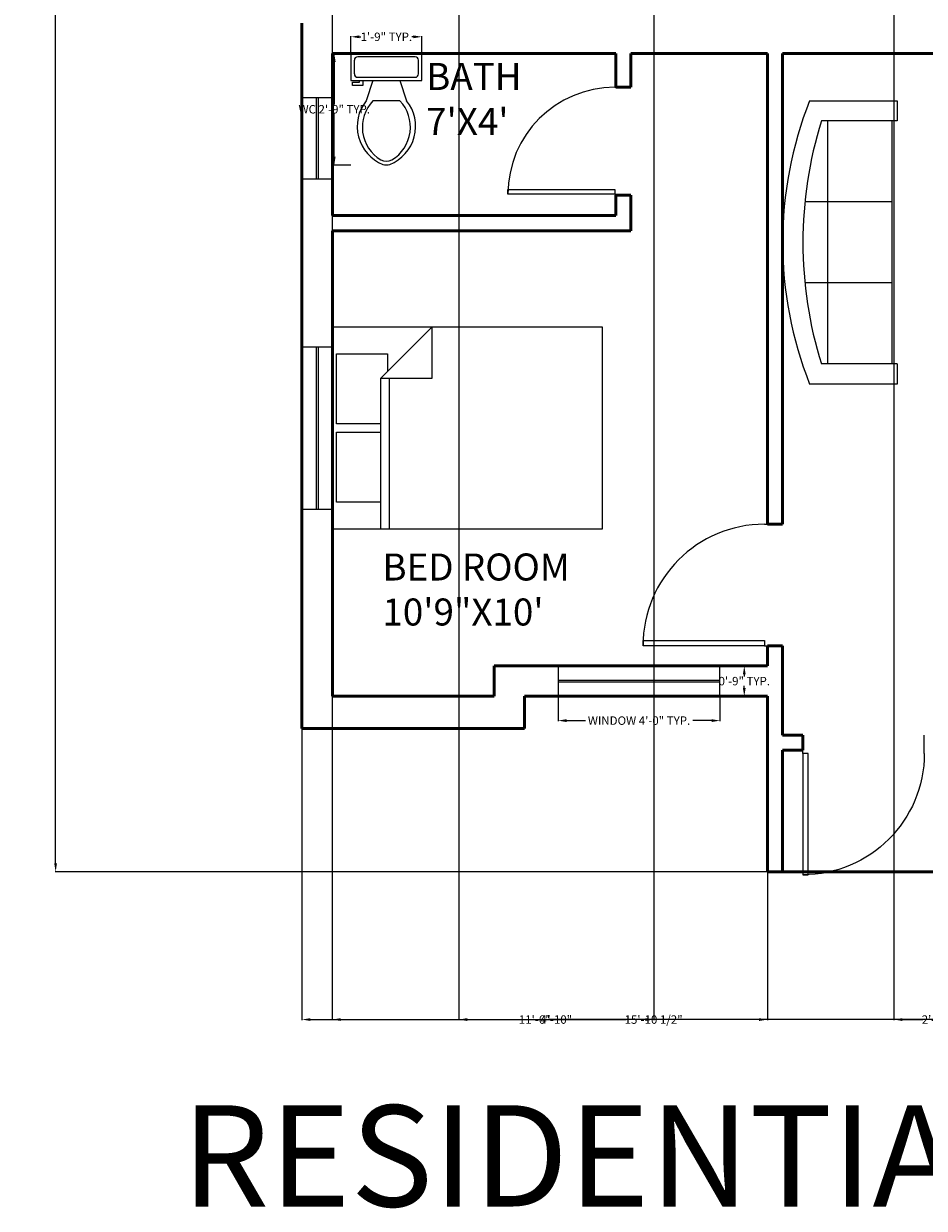
# Model space of a CAD drawing. Units: inches. Extents: x -46 to 565, y -56 to 809.
# Tile 1 of 6: x -46 to 221, y -56 to 296. Entities that reach past the tile are written whole.
import ezdxf

# ---------------------------------------------------------------- set-up
doc = ezdxf.new("R2010")
doc.units = ezdxf.units.IN
doc.header["$MEASUREMENT"] = 0
for name, color, linetype, lineweight in [('A-ANNO-DIMS', 2, 'Continuous', 18), ('A-ANNO-TEXT', 241, 'Continuous', 30), ('A-AREA-IDEN', 241, 'Continuous', 18), ('A-FLOR-FIXT', 131, 'Continuous', 18), ('A-FURN', 131, 'Continuous', 18), ('DOOR', 210, 'Continuous', 25), ('WALL', 10, 'Continuous', 50), ('WINDOW', 170, 'Continuous', 18)]:
    doc.layers.add(name, color=color, linetype=linetype, lineweight=lineweight)
doc.styles.get("Standard").update_dxf_attribs({"font": 'arial.ttf'})
doc.dimstyles.get("Standard").update_dxf_attribs({"dimtxt": 2.5, "dimasz": 2.5, "dimexe": 0.18, "dimexo": 0.0625, "dimgap": 0.09, "dimtad": 0, "dimtih": 1, "dimtoh": 1, "dimzin": 0, "dimdsep": 46, "dimlunit": 3, "dimtxsty": 'Standard', "dimcen": 0.09, "dimadec": 0, "dimazin": 0, "dimtfac": 1, "dimtofl": 0, "dimtmove": 0, "dimatfit": 3, "dimfxl": 1, "dimtolj": 1, "dimtzin": 0, "dimarcsym": 0})

# ---------------------------------------------------------------- blocks, each defined once
blk = doc.blocks.new('*U2')
for p, q in [((0, 0), (0, -6)), ((40, 0), (40, -6))]:
    blk.add_line(p, q)
blk.add_lwpolyline([(0, 0), (0, 40), (1.75, 40), (1.75, 0)], close=True)
blk.add_arc((0, 0), 40, 0, 90)
blk = doc.blocks.new('Bed - Queen')
for p, q in [((0, -80.00003), (0, 0)), ((0, 0), (59.99999, 0)), ((59.99999, 0), (59.99999, -80.00003)), ((7.99999, -1.2), (28.79998, -1.2)), ((7.99999, -14.4), (7.99999, -1.2)), ((28.79998, -1.2), (28.79998, -14.4)), ((31.19999, -1.2), (51.99999, -1.2)), ((31.19999, -14.4), (31.19999, -1.2)), ((51.99999, -1.2), (51.99999, -16.4)), ((0, -14.4), (44.8, -14.4)), ((44.8, -16.8), (0, -16.8)), ((59.99999, -29.6), (44.8, -14.4)), ((44.8, -14.4), (44.8, -29.6)), ((51.99999, -16.4), (46.79936, -16.4)), ((44.8, -29.6), (59.99999, -29.6)), ((59.99999, -80.00003), (0, -80.00003))]:
    blk.add_line(p, q)
blk = doc.blocks.new('Toilet - top')
for p, q in [((9.5, -6), (9.5, -2)), ((-10, -8.5), (-8, -8.5)), ((-10, -9.5), (-10, -8.5)), ((-7, -9.5), (-10, -9.5)), ((-8, -8.5), (-8, -8)), ((-7, -8), (-7, -9.5)), ((-4, -8), (-6, -14)), ((4, -8), (6, -14)), ((4, -14), (-4, -14))]:
    blk.add_line(p, q)
blk.add_lwpolyline([(10.5, -8), (10.5, 0), (-10.5, 0), (-10.5, -8)], close=True)
for points in [[(-9.5, -2), (-9.5, -6)], [(8.5, -1), (-8.5, -1)], [(-8.5, -7), (8.5, -7)]]:
    blk.add_lwpolyline(points)
for centre, radius, start, end in [((-8.62, -1.88), 0.884, 81.8699, 188.1301), ((8.62, -1.88), 0.884, 351.8699, 98.1301), ((-8.62, -6.12), 0.884, 171.8699, 278.1301), ((8.62, -6.12), 0.884, 261.8699, 8.1301), ((3.52, -21.58), 12.17, 141.4691, 247.9714), ((4.2, -21.82), 11.33, 136.3677, 238.9468), ((-3.52, -21.58), 12.17, 292.0284, 38.5307), ((-4.2, -21.82), 11.33, 301.053, 43.6321), ((0, -27.88), 4, 245.7318, 294.2682), ((0, -29), 4, 254.8605, 285.1395)]:
    blk.add_arc(centre, radius, start, end)
blk = doc.blocks.new('Sofa - Roundback 7 ft.')
for p, q in [((-12.00002, -32.4421), (-12.00003, -6.5971)), ((11.99997, -32.4421), (11.99998, -6.5971)), ((-36.000027, -34), (-36.000027, -11.4696)), ((-35.999844, -13.3819), (35.9998, -13.3819)), ((35.99998, -34), (35.99998, -11.4696)), ((-36.000027, -32.4421), (35.99998, -32.4421))]:
    blk.add_line(p, q)
for points in [[(-36.000027, -34), (-42.000027, -34), (-42.000027, -8)], [(41.99998, -8), (41.99998, -34), (35.99998, -34)]]:
    blk.add_lwpolyline(points)
for centre, radius, start, end in [((0, -114.25), 114.25, 68.43141, 111.5686), ((-0.00001, -127.1968), 121.1968, 72.72033, 107.2797)]:
    blk.add_arc(centre, radius, start, end)
blk = doc.blocks.new('*D15')
at = {"layer": 'A-ANNO-DIMS', "color": 0, "lineweight": -2, "transparency": 16777216}
for p, q in [((174.08, 764.2), (-37.07, 764.2)), ((-36.89, 761.7), (-36.89, 409.4)), ((-36.89, 46.7), (-36.89, 399)), ((174.08, 44.2), (-37.07, 44.2))]:
    blk.add_line(p, q, dxfattribs=at)
at = {"layer": 'A-ANNO-DIMS', "color": 0, "transparency": 16777216}
for points in [[(-37.31, 761.7), (-36.48, 761.7), (-36.89, 764.2)], [(-37.31, 46.7), (-36.48, 46.7), (-36.89, 44.2)]]:
    blk.add_solid(points, dxfattribs=at)
at = {"layer": 'Defpoints', "color": 0, "transparency": 16777216}
for p in [(-36.89, 764.2), (174.14, 764.2), (174.14, 44.2)]:
    blk.add_point(p, dxfattribs=at)
at = {"layer": 'A-ANNO-DIMS', "color": 0, "transparency": 16777216, "insert": (-36.89, 404.2), "char_height": 10, "attachment_point": 5}
blk.add_mtext("\\A1;60'", dxfattribs=at)
blk = doc.blocks.new('WIN-48IN')
for p, q in [((0, 4.75), (48, 4.75)), ((0, 4.25), (48, 4.25))]:
    blk.add_line(p, q)
blk.add_lwpolyline([(0, 0), (48, 0), (48, 9), (0, 9)], close=True)
blk = doc.blocks.new('WIN-24IN')
for p, q in [((4.25, 24), (4.25, 0)), ((4.75, 24), (4.75, 0))]:
    blk.add_line(p, q)
blk.add_lwpolyline([(0, 24), (0, 0), (9, 0), (9, 24)], close=True)
blk = doc.blocks.new('*D21')
at = {"layer": 'A-ANNO-DIMS', "color": 0, "lineweight": -2, "transparency": 16777216}
for p, q in [((50.6, 286.7), (45.53, 286.7)), ((45.71, 284.2), (45.71, 271.56)), ((45.71, 256.15), (45.71, 268.79)), ((50.6, 253.65), (45.53, 253.65))]:
    blk.add_line(p, q, dxfattribs=at)
at = {"layer": 'A-ANNO-DIMS', "color": 0, "transparency": 16777216}
for points in [[(45.29, 284.2), (46.12, 284.2), (45.71, 286.7)], [(45.29, 256.15), (46.12, 256.15), (45.71, 253.65)]]:
    blk.add_solid(points, dxfattribs=at)
at = {"layer": 'Defpoints', "color": 0, "transparency": 16777216}
for p in [(45.71, 286.7), (50.66, 286.7), (50.66, 253.65)]:
    blk.add_point(p, dxfattribs=at)
at = {"layer": 'A-ANNO-DIMS', "color": 0, "transparency": 16777216, "insert": (45.71, 270.18), "char_height": 2.5, "attachment_point": 5}
blk.add_mtext('\\A1;WC 2\'-9" TYP.', dxfattribs=at)
blk = doc.blocks.new('*D22')
at = {"layer": 'A-ANNO-DIMS', "color": 0, "lineweight": -2, "transparency": 16777216}
for p, q in [((50.66, 286.76), (50.66, 291.84)), ((53.16, 291.66), (53.57, 291.66)), ((69.16, 291.66), (68.75, 291.66)), ((71.66, 286.76), (71.66, 291.84))]:
    blk.add_line(p, q, dxfattribs=at)
at = {"layer": 'A-ANNO-DIMS', "color": 0, "transparency": 16777216}
for points in [[(53.16, 292.07), (53.16, 291.24), (50.66, 291.66)], [(69.16, 292.07), (69.16, 291.24), (71.66, 291.66)]]:
    blk.add_solid(points, dxfattribs=at)
at = {"layer": 'Defpoints', "color": 0, "transparency": 16777216}
for p in [(71.66, 291.66), (50.66, 286.7), (71.66, 286.7)]:
    blk.add_point(p, dxfattribs=at)
at = {"layer": 'A-ANNO-DIMS', "color": 0, "transparency": 16777216, "insert": (61.16, 291.66), "char_height": 2.5, "attachment_point": 5}
blk.add_mtext('\\A1;1\'-9" TYP.', dxfattribs=at)
blk = doc.blocks.new('*D23')
at = {"layer": 'A-ANNO-DIMS', "color": 0, "lineweight": -2, "transparency": 16777216}
for p, q in [((112.07, 96.14), (112.07, 88.82)), ((160.07, 96.14), (160.07, 88.82)), ((114.57, 89), (120.16, 89)), ((157.57, 89), (151.97, 89))]:
    blk.add_line(p, q, dxfattribs=at)
at = {"layer": 'A-ANNO-DIMS', "color": 0, "transparency": 16777216}
for points in [[(114.57, 89.42), (114.57, 88.58), (112.07, 89)], [(157.57, 89.42), (157.57, 88.58), (160.07, 89)]]:
    blk.add_solid(points, dxfattribs=at)
at = {"layer": 'Defpoints', "color": 0, "transparency": 16777216}
for p in [(112.07, 96.2), (160.07, 96.2), (160.07, 89)]:
    blk.add_point(p, dxfattribs=at)
at = {"layer": 'A-ANNO-DIMS', "color": 0, "transparency": 16777216, "insert": (136.07, 89), "char_height": 2.5, "attachment_point": 5}
blk.add_mtext('\\A1;WINDOW 4\'-0" TYP.', dxfattribs=at)
blk = doc.blocks.new('*D24')
at = {"layer": 'A-ANNO-DIMS', "color": 0, "lineweight": -2, "transparency": 16777216}
for p, q in [((160.13, 105.2), (167.45, 105.2)), ((167.27, 102.7), (167.27, 102.07)), ((167.27, 98.7), (167.27, 99.33)), ((160.13, 96.2), (167.45, 96.2))]:
    blk.add_line(p, q, dxfattribs=at)
at = {"layer": 'A-ANNO-DIMS', "color": 0, "transparency": 16777216}
for points in [[(166.85, 102.7), (167.68, 102.7), (167.27, 105.2)], [(166.85, 98.7), (167.68, 98.7), (167.27, 96.2)]]:
    blk.add_solid(points, dxfattribs=at)
at = {"layer": 'Defpoints', "color": 0, "transparency": 16777216}
for p in [(160.07, 105.2), (167.27, 105.2), (160.07, 96.2)]:
    blk.add_point(p, dxfattribs=at)
at = {"layer": 'A-ANNO-DIMS', "color": 0, "transparency": 16777216, "insert": (167.27, 100.7), "char_height": 2.5, "attachment_point": 5}
blk.add_mtext('\\A1;0\'-9" TYP.', dxfattribs=at)
blk = doc.blocks.new('*D48')
at = {"layer": 'A-ANNO-DIMS', "color": 0, "lineweight": -2, "transparency": 16777216}
for p, q in [((36.14, 86.62), (36.14, 0.22)), ((174.14, 44.14), (174.14, 0.22)), ((38.64, 0.4), (100.88, 0.4)), ((171.64, 0.4), (109.41, 0.4))]:
    blk.add_line(p, q, dxfattribs=at)
at = {"layer": 'A-ANNO-DIMS', "color": 0, "transparency": 16777216}
for points in [[(38.64, 0.82), (38.64, -0.02), (36.14, 0.4)], [(171.64, 0.82), (171.64, -0.02), (174.14, 0.4)]]:
    blk.add_solid(points, dxfattribs=at)
at = {"layer": 'Defpoints', "color": 0, "transparency": 16777216}
for p in [(36.14, 86.68), (174.14, 44.2), (174.14, 0.4)]:
    blk.add_point(p, dxfattribs=at)
at = {"layer": 'A-ANNO-DIMS', "color": 0, "transparency": 16777216, "insert": (105.14, 0.4), "char_height": 2.5, "attachment_point": 5}
blk.add_mtext('\\A1;11\'-6"', dxfattribs=at)
blk = doc.blocks.new('*D50')
at = {"layer": 'A-ANNO-DIMS', "color": 0, "lineweight": -2, "transparency": 16777216}
for p, q in [((211.64, 558.64), (211.64, 0.22)), ((235.64, 558.64), (235.64, 0.22)), ((214.14, 0.4), (220.21, 0.4)), ((233.14, 0.4), (227.08, 0.4))]:
    blk.add_line(p, q, dxfattribs=at)
at = {"layer": 'A-ANNO-DIMS', "color": 0, "transparency": 16777216}
for points in [[(214.14, 0.82), (214.14, -0.02), (211.64, 0.4)], [(233.14, 0.82), (233.14, -0.02), (235.64, 0.4)]]:
    blk.add_solid(points, dxfattribs=at)
at = {"layer": 'Defpoints', "color": 0, "transparency": 16777216}
for p in [(211.64, 558.7), (235.64, 558.7), (235.64, 0.4)]:
    blk.add_point(p, dxfattribs=at)
at = {"layer": 'A-ANNO-DIMS', "color": 0, "transparency": 16777216, "insert": (223.64, 0.4), "char_height": 2.5, "attachment_point": 5}
blk.add_mtext('\\A1;2\'-0"', dxfattribs=at)
blk = doc.blocks.new('*D51')
at = {"layer": 'A-ANNO-DIMS', "color": 0, "lineweight": -2, "transparency": 16777216}
for p, q in [((82.64, 554.14), (82.64, 0.22)), ((140.42, 554.14), (140.42, 0.22)), ((85.14, 0.4), (107.1, 0.4)), ((137.92, 0.4), (115.96, 0.4))]:
    blk.add_line(p, q, dxfattribs=at)
at = {"layer": 'A-ANNO-DIMS', "color": 0, "transparency": 16777216}
for points in [[(85.14, 0.82), (85.14, -0.02), (82.64, 0.4)], [(137.92, 0.82), (137.92, -0.02), (140.42, 0.4)]]:
    blk.add_solid(points, dxfattribs=at)
at = {"layer": 'Defpoints', "color": 0, "transparency": 16777216}
for p in [(82.64, 554.2), (140.42, 554.2), (140.42, 0.4)]:
    blk.add_point(p, dxfattribs=at)
at = {"layer": 'A-ANNO-DIMS', "color": 0, "transparency": 16777216, "insert": (111.53, 0.4), "char_height": 2.5, "attachment_point": 5}
blk.add_mtext('\\A1;4\'-10"', dxfattribs=at)
blk = doc.blocks.new('*D55')
at = {"layer": 'A-ANNO-DIMS', "color": 0, "lineweight": -2, "transparency": 16777216}
for p, q in [((45.14, 407.14), (45.14, 0.22)), ((235.64, 407.14), (235.64, 0.22)), ((47.64, 0.4), (132.24, 0.4)), ((233.14, 0.4), (148.54, 0.4))]:
    blk.add_line(p, q, dxfattribs=at)
at = {"layer": 'A-ANNO-DIMS', "color": 0, "transparency": 16777216}
for points in [[(47.64, 0.82), (47.64, -0.02), (45.14, 0.4)], [(233.14, 0.82), (233.14, -0.02), (235.64, 0.4)]]:
    blk.add_solid(points, dxfattribs=at)
at = {"layer": 'Defpoints', "color": 0, "transparency": 16777216}
for p in [(45.14, 407.2), (235.64, 407.2), (235.64, 0.4)]:
    blk.add_point(p, dxfattribs=at)
at = {"layer": 'A-ANNO-DIMS', "color": 0, "transparency": 16777216, "insert": (140.39, 0.4), "char_height": 2.5, "attachment_point": 5}
blk.add_mtext('\\A1;15\'-10 1/2"', dxfattribs=at)

msp = doc.modelspace()

# ---------------------------------------------------------------- linework, layer by layer
at = {"layer": 'WALL'}
for p, q in [((36.143, 295.7), (36.143, 86.684)), ((45.143, 286.7), (45.143, 238.7)), ((129.143, 286.7), (45.143, 286.7)), ((129.143, 286.7), (129.143, 276.7)), ((133.643, 286.7), (133.643, 276.7)), ((174.143, 286.7), (133.643, 286.7)), ((174.143, 286.7), (174.143, 147.2)), ((244.643, 286.7), (178.643, 286.7)), ((178.643, 286.7), (178.643, 147.2)), ((133.643, 276.7), (129.143, 276.7)), ((133.643, 244.7), (129.143, 244.7)), ((129.143, 244.7), (129.143, 238.7)), ((133.643, 244.7), (133.643, 234.2)), ((129.143, 238.7), (45.143, 238.7)), ((45.143, 234.2), (45.143, 114.2)), ((133.643, 234.2), (45.143, 234.2)), ((174.143, 147.2), (178.643, 147.2)), ((45.143, 114.2), (45.143, 96.2)), ((174.143, 111.2), (178.643, 111.2)), ((174.143, 111.2), (174.143, 105.2)), ((178.643, 111.2), (178.643, 96.2)), ((102.143, 105.2), (93.143, 105.2)), ((93.143, 105.2), (93.143, 96.2)), ((174.143, 105.2), (102.143, 105.2)), ((93.143, 96.2), (45.143, 96.2)), ((174.143, 96.2), (102.143, 96.2)), ((129.143, 96.2), (102.143, 96.2)), ((102.143, 96.2), (102.143, 86.684)), ((174.143, 44.2), (174.143, 96.2)), ((178.643, 96.2), (178.643, 84.7)), ((102.143, 86.684), (36.143, 86.684)), ((184.643, 84.7), (178.643, 84.7)), ((184.643, 84.7), (184.643, 80.2)), ((184.643, 80.2), (178.643, 80.2)), ((178.643, 80.2), (178.643, 44.2)), ((235.643, 44.2), (174.143, 44.2))]:
    msp.add_line(p, q, dxfattribs=at)

# ---------------------------------------------------------------- block references
at = {"layer": 'A-FLOR-FIXT'}
msp.add_blockref('Toilet - top', (61.163, 286.7), dxfattribs=at)
at = {"layer": 'A-FURN', "rotation": 90}
for name, p in [('Sofa - Roundback 7 ft.', (178.643, 230.706)), ('Bed - Queen', (45.143, 145.711))]:
    msp.add_blockref(name, p, dxfattribs=at)
at = {"layer": 'DOOR'}
for p, xscale, yscale, zscale, rotation in [((128.887, 244.991), 0.7927140230435884, 0.7927140230435884, 0.7927140230435884, 90), ((173.243, 111.2), 0.9, 0.9, 0.9, 90), ((184.643, 79.3), -0.8999999999999971, 0.8999999999999971, 0.8999999999999971, 180)]:
    msp.add_blockref('*U2', p, dxfattribs=dict(at, xscale=xscale, yscale=yscale, zscale=zscale, rotation=rotation))
at = {"layer": 'WINDOW'}
for name, p in [('WIN-24IN', (36.143, 249.565)), ('WIN-48IN', (112.066, 96.2))]:
    msp.add_blockref(name, p, dxfattribs=at)
at = {"layer": 'WINDOW', "rotation": 269.9999999999999}
msp.add_blockref('WIN-48IN', (36.143, 199.711), dxfattribs=at)

# ---------------------------------------------------------------- texts
at = {"layer": 'A-ANNO-TEXT', "insert": (0.465, -25.004), "char_height": 30, "attachment_point": 1}
msp.add_mtext_dynamic_manual_height_columns('RESIDENTIAL FLOOR PLAN', width=551.91415, gutter_width=1, heights=[0], dxfattribs=at)
at = {"layer": 'A-AREA-IDEN', "char_height": 8, "attachment_point": 1}
for s, insert in [("BATH\\P7'X4' ", (72.949, 283.905)), ('BED ROOM\\P10\'9"X10\'', (59.986, 138.523))]:
    msp.add_mtext_dynamic_manual_height_columns(s, width=70.77133, gutter_width=1, heights=[0], dxfattribs=dict(at, insert=insert))

# ---------------------------------------------------------------- dimensions: what is measured, and where the dimension line sits
at = {"layer": 'A-ANNO-DIMS'}
dim = msp.add_aligned_dim(p1=(174.143, 44.2), p2=(174.143, 764.2), distance=211.037, dimstyle='Standard', override={"dimtxt": 10, "dimclrd": 0, "dimclre": 0, "dimclrt": 0}, dxfattribs=at)
dim.commit()
dim.dimension.update_dxf_attribs({"geometry": '*D15', "text_midpoint": (-36.894, 404.2)})
for base, p1, p2, picture, middle in [((235.643, 0.4), (211.643, 558.7), (235.643, 558.7), '*D50', (223.643, 0.4)), ((140.418, 0.4), (82.643, 554.2), (140.418, 554.2), '*D51', (111.53, 0.4)), ((235.643, 0.4), (45.143, 407.2), (235.643, 407.2), '*D55', (140.393, 0.4)), ((174.143, 0.4), (36.143, 86.684), (174.143, 44.2), '*D48', (105.143, 0.4))]:
    dim = msp.add_linear_dim(base=base, p1=p1, p2=p2, dimstyle='Standard', override={"dimdec": 1, "dimlfac": 1, "dimrnd": 0, "dimzin": 1, "dimdsep": 46, "dimlunit": 4, "dimfrac": 2}, dxfattribs=at)
    dim.commit()
    dim.dimension.update_dxf_attribs({"geometry": picture, "text_midpoint": middle})
for base, p1, p2, text, picture, middle in [((71.663, 291.657), (50.663, 286.7), (71.663, 286.7), '<> TYP.', '*D22', (61.163, 291.657)), ((160.066, 89), (112.066, 96.2), (160.066, 96.2), 'WINDOW <> TYP.', '*D23', (136.066, 89))]:
    dim = msp.add_linear_dim(base=base, p1=p1, p2=p2, text=text, dimstyle='Standard', override={"dimdec": 1, "dimlfac": 1, "dimrnd": 0, "dimzin": 1, "dimdsep": 46, "dimlunit": 4, "dimfrac": 2}, dxfattribs=at)
    dim.commit()
    dim.dimension.update_dxf_attribs({"geometry": picture, "text_midpoint": middle})
for base, p1, p2, text, picture, middle in [((45.706, 286.7), (50.663, 253.653), (50.663, 286.7), 'WC <> TYP.', '*D21', (45.706, 270.177)), ((167.266, 105.2), (160.066, 96.2), (160.066, 105.2), '<> TYP.', '*D24', (167.266, 100.7))]:
    dim = msp.add_linear_dim(base=base, p1=p1, p2=p2, angle=90, text=text, dimstyle='Standard', override={"dimdec": 1, "dimlfac": 1, "dimrnd": 0, "dimzin": 1, "dimdsep": 46, "dimlunit": 4, "dimfrac": 2}, dxfattribs=at)
    dim.commit()
    dim.dimension.update_dxf_attribs({"geometry": picture, "text_midpoint": middle})

doc.saveas('drawing.dxf')
